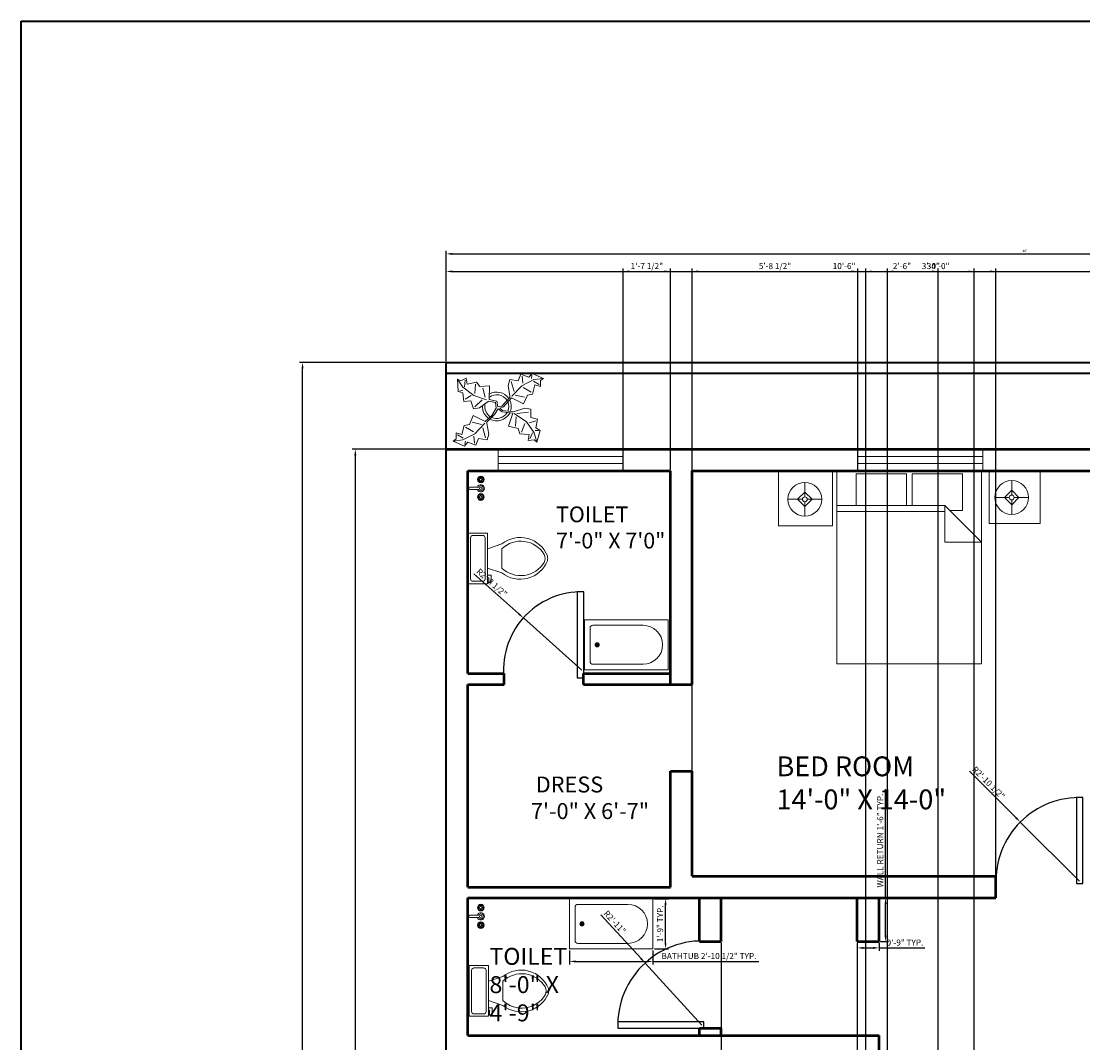
# Model space of a CAD drawing. Units: inches. Extents: x 65 to 818, y -87 to 880.
# Tile 5 of 6: x 65 to 505, y 457 to 880. Entities that reach past the tile are written whole.
import ezdxf

# ---------------------------------------------------------------- set-up
doc = ezdxf.new("R2010")
doc.units = ezdxf.units.IN
for name, color, linetype, lineweight in [('A-ANNO-DIMS', 2, 'Continuous', 18), ('A-ANNO-TTLB', 7, 'Continuous', 35), ('A-AREA-IDEN', 7, 'Continuous', 25), ('A-DOOR', 3, 'Continuous', 25), ('A-FLOR-FIXT', 9, 'Continuous', 18), ('A-FURN', 8, 'Continuous', 18), ('A-GLAZ', 4, 'Continuous', 18), ('A-WALL', 7, 'Continuous', 50), ('C-PROP', 7, 'Continuous', 35), ('E-LITE', 2, 'Continuous', 18), ('L-PLNT', 94, 'Continuous', 13)]:
    doc.layers.add(name, color=color, linetype=linetype, lineweight=lineweight)
doc.styles.get("Standard").update_dxf_attribs({"font": 'arial.ttf'})
doc.dimstyles.new('ISO-25', dxfattribs={"dimtxt": 2.5, "dimasz": 2.5, "dimexe": 1.25, "dimexo": 0.625, "dimtad": 1, "dimtxsty": 'Standard', "dimcen": 2.5, "dimadec": 0, "dimazin": 0, "dimtfac": 1, "dimtmove": 0, "dimatfit": 3, "dimfxl": 1, "dimarcsym": 0})

# ---------------------------------------------------------------- blocks, each defined once
blk = doc.blocks.new('Bed - Queen')
for p, q in [((0, -80.00003), (0, 0)), ((0, 0), (59.99999, 0)), ((59.99999, 0), (59.99999, -80.00003)), ((7.99999, -1.2), (28.79998, -1.2)), ((7.99999, -14.4), (7.99999, -1.2)), ((28.79998, -1.2), (28.79998, -14.4)), ((31.19999, -1.2), (51.99999, -1.2)), ((31.19999, -14.4), (31.19999, -1.2)), ((51.99999, -1.2), (51.99999, -16.4)), ((0, -14.4), (44.8, -14.4)), ((44.8, -16.8), (0, -16.8)), ((59.99999, -29.6), (44.8, -14.4)), ((44.8, -14.4), (44.8, -29.6)), ((51.99999, -16.4), (46.79936, -16.4)), ((44.8, -29.6), (59.99999, -29.6)), ((59.99999, -80.00003), (0, -80.00003))]:
    blk.add_line(p, q)
blk = doc.blocks.new('Toilet - top')
for p, q in [((9.5, -6), (9.5, -2)), ((-10, -8.5), (-8, -8.5)), ((-10, -9.5), (-10, -8.5)), ((-8, -8.5), (-8, -8)), ((-7, -8), (-7, -9.5)), ((-4, -8), (-6, -14)), ((4, -8), (6, -14)), ((-7, -9.5), (-10, -9.5)), ((4, -14), (-4, -14))]:
    blk.add_line(p, q)
blk.add_lwpolyline([(10.5, -8), (10.5, 0), (-10.5, 0), (-10.5, -8)], close=True)
for points in [[(-9.5, -2), (-9.5, -6)], [(8.5, -1), (-8.5, -1)], [(-8.5, -7), (8.5, -7)]]:
    blk.add_lwpolyline(points)
for centre, radius, start, end in [((-8.62, -1.88), 0.884, 81.8699, 188.1301), ((8.62, -1.88), 0.884, 351.8699, 98.1301), ((-8.62, -6.12), 0.884, 171.8699, 278.1301), ((8.62, -6.12), 0.884, 261.8699, 8.1301), ((3.52, -21.58), 12.17, 141.4691, 247.9714), ((4.2, -21.82), 11.33, 136.3677, 238.9468), ((-3.52, -21.58), 12.17, 292.0284, 38.5307), ((-4.2, -21.82), 11.33, 301.053, 43.6321), ((0, -27.88), 4, 245.7318, 294.2682), ((0, -29), 4, 254.8605, 285.1395)]:
    blk.add_arc(centre, radius, start, end)
blk = doc.blocks.new('Bath Tub - 26 x 60 in.')
for p, q in [((8, -18), (10, -18)), ((9, -17), (9, -19))]:
    blk.add_line(p, q)
blk.add_lwpolyline([(0, -36), (0, 0), (60, 0), (60, -36)], close=True)
for points in [[(4, -30), (4, -6)], [(6, -4), (42, -4)], [(42, -32), (6, -32)]]:
    blk.add_lwpolyline(points)
for radius in [1.5, 1]:
    blk.add_circle((9, -18), radius)
for centre, radius, start, end in [((5.75, -5.75), 1.77, 81.8699, 188.1301), ((42, -18), 14, 270, 90), ((5.75, -30.25), 1.77, 171.8699, 278.1301)]:
    blk.add_arc(centre, radius, start, end)
blk = doc.blocks.new('Faucet - Bathroom top')
for p, q in [((-4.107, 0.125), (-4.375, 0.125)), ((-3.75, 0.4788), (-3.75, 0.75)), ((-3.5, 0.482), (-3.5, 0.75)), ((-3.1461, 0.125), (-2.875, 0.125)), ((3.143, 0.125), (2.875, 0.125)), ((3.5, 0.4788), (3.5, 0.75)), ((3.75, 0.482), (3.75, 0.75)), ((4.1039, 0.125), (4.375, 0.125)), ((-4.1039, -0.125), (-4.375, -0.125)), ((-3.75, -0.4821), (-3.75, -0.75)), ((-3.5, -0.4789), (-3.5, -0.75)), ((-3.143, -0.125), (-2.875, -0.125)), ((-0.5, -0.8639), (-0.5, -4.5)), ((0.5, -4.5), (0.5, -0.8631)), ((3.1461, -0.125), (2.875, -0.125)), ((3.5, -0.4821), (3.5, -0.75)), ((3.75, -0.4789), (3.75, -0.75)), ((4.107, -0.125), (4.375, -0.125))]:
    blk.add_line(p, q)
for centre, radius in [((-3.625, 0), 1.375), ((-4.625, 0), 0.2795), ((-3.625, 0), 0.5), ((-3.625, 1), 0.2795), ((-2.625, 0), 0.2795), ((0, 0), 0.5), ((3.625, 0), 1.375), ((2.625, 0), 0.2795), ((3.625, 0), 0.5), ((3.625, 1), 0.2795), ((4.625, 0), 0.2795), ((-3.625, -1), 0.2795), ((3.625, -1), 0.2795)]:
    blk.add_circle(centre, radius)
for centre, radius, start, end in [((-3.625, 0), 1, 105.2407, 164.2093), ((-3.625, 0), 1, 16.44125, 74.07887), ((0, 0), 1.5, 289.6514, 250.3603), ((0, 0), 1, 300.3431, 239.7554), ((3.625, 0), 1, 106.12, 164.0884), ((3.625, 0), 1, 16.23422, 73.90469), ((-3.625, 0), 1, 196.2342, 253.9047), ((-3.625, 0), 1, 286.12, 344.0884), ((3.625, 0), 1, 196.4413, 254.0789), ((3.625, 0), 1, 285.2407, 344.2093), ((0, -4.5), 0.5, 180, 0)]:
    blk.add_arc(centre, radius, start, end)
blk = doc.blocks.new('Plant - Rubber or Philodendron')
for p, q in [((8.8871, 10.7908), (9.9809, 13.4933)), ((9.9809, 13.4933), (13.3837, 12.301)), ((13.3837, 12.301), (14.68, 13.9039)), ((14.68, 13.9039), (19.3848, 11.8146)), ((-16.2005, 11.4774), (-13.9899, 8.1064)), ((-16.2005, 11.4774), (-14.8639, 10.7964)), ((-16.0159, 6.3329), (-16.2005, 11.4774)), ((-14.8639, 10.7964), (-12.6195, 11.8975)), ((-13.3174, 8.325), (-13.0735, 11.0065)), ((-12.6195, 11.8975), (-12.1909, 9.4345)), ((-12.1909, 9.4345), (-8.3829, 10.3)), ((-8.8369, 9.409), (-9.0894, 5.6095)), ((-8.3829, 10.3), (-7.0549, 8.501)), ((4.6914, 8.8812), (5.3859, 11.2828)), ((4.6914, 8.8812), (5.5014, 4.4831)), ((5.3859, 11.2828), (8.8871, 10.7908)), ((5.9878, 10.4842), (7.1971, 6.3869)), ((15.3859, 11.3055), (10.3916, 8.7942)), ((10.5828, 12.6946), (10.8893, 9.7953)), ((14.5816, 13.2037), (14.3848, 11.8033)), ((15.7909, 9.1065), (14.8995, 5.3044)), ((15.2875, 10.6053), (17.5907, 9.2105)), ((19.3848, 11.8146), (15.3859, 11.3055)), ((18.1925, 8.4119), (15.7909, 9.1065)), ((19.3848, 11.8146), (18.1868, 10.9119)), ((18.1868, 10.9119), (18.1925, 8.4119)), ((-14.0069, 5.8704), (-16.0159, 6.3329)), ((-15.3434, 6.5514), (-13.9984, 6.9884)), ((-13.5868, 2.2894), (-14.0069, 5.8704)), ((-13.9899, 8.1064), (-9.5434, 4.7185)), ((-13.1329, 3.1804), (-10.6614, 4.727)), ((-9.5434, 4.7185), (-4.1917, 2.9888)), ((-7.0549, 8.501), (-3.0284, 8.6941)), ((-4.8529, 4.012), (-5.7184, 7.82)), ((-3.0284, 8.6941), (-3.0709, 3.1041)), ((5.4346, 3.9146), (5.5014, 4.4831)), ((10.3916, 8.7942), (6.2847, 4.4028)), ((7.7005, 4.8881), (11.5025, 3.9967)), ((14.2977, 6.1031), (10.9934, 7.9956)), ((12.7005, 4.8994), (11.1089, 1.1958)), ((14.8995, 5.3044), (12.7005, 4.8994)), ((-10.6784, 2.491), (-13.5868, 2.2894)), ((-9.5858, -0.8715), (-10.6784, 2.491)), ((-9.1318, 0.0195), (-5.9793, 2.9025)), ((-7.1228, -0.443), (-3.5248, 2.2131)), ((-3.5248, 2.2131), (-3.3011, 2.4355)), ((-3.3011, 2.4355), (-0.5306, 1.7947)), ((-3.0709, 3.1041), (0.0797, 2.3163)), ((-0.5306, 1.7947), (-0.2255, -0.5527)), ((-0.5306, 1.7947), (-0.5306, 1.7947)), ((0.0797, 2.3163), (0.4866, -0.031)), ((0.4866, -0.031), (2.1141, 0.2298)), ((2.1141, 0.2298), (5.4346, 3.9146)), ((6.1032, 3.6844), (2.8262, -0.031)), ((11.1089, 1.1958), (6.1032, 3.6844)), ((-11.3237, -7.2629), (-9.7321, -3.5593)), ((-9.7321, -3.5593), (-4.7264, -6.0479)), ((-7.1228, -0.443), (-9.5858, -0.8715)), ((-2.019, -3.6148), (-4.7264, -6.0479)), ((-4.0579, -6.2781), (-0.9375, -3.1608)), ((-2.019, -3.6148), (-0.2255, -0.5527)), ((-0.9375, -3.1608), (0.5883, -0.8135)), ((0.5883, -0.8135), (2.2447, -2.0916)), ((2.8262, -0.031), (1.3003, -0.5527)), ((1.3003, -0.5527), (2.4193, -1.4655)), ((2.2447, -2.0916), (6.7108, -2.6626)), ((2.4193, -1.4655), (6.895, -2.1175)), ((4.943, -7.9659), (6.7108, -2.6626)), ((11.6605, -0.5413), (6.895, -2.1175)), ((12.3677, -6.1981), (7.219, -2.6772)), ((8.125, -4.0768), (7.7715, -7.9659)), ((8.3544, -2.7453), (13.1973, -2.1704)), ((11.6605, -0.5413), (14.1354, -0.8948)), ((14.1354, -0.8948), (14.1354, -4.4304)), ((-14.4141, -11.4699), (-13.5228, -7.6679)), ((-13.5228, -7.6679), (-11.3237, -7.2629)), ((-12.921, -8.4665), (-9.6166, -10.359)), ((-6.3237, -7.2516), (-10.1257, -6.3602)), ((-9.0148, -11.1577), (-4.9047, -6.8122)), ((-4.611, -12.8477), (-5.8203, -8.7504)), ((-4.1246, -6.8466), (-4.0579, -6.2781)), ((-3.3146, -11.2447), (-4.1246, -6.8466)), ((8.8321, -9.0266), (4.943, -7.9659)), ((10.2463, -10.4408), (11.6605, -6.9053)), ((15.5496, -10.7943), (12.3677, -6.1981)), ((16.2567, -5.8446), (13.4283, -6.5517)), ((14.1354, -4.4304), (16.9638, -5.1375)), ((16.9638, -5.1375), (16.2567, -8.673)), ((16.2567, -8.673), (18.0245, -9.7337)), ((-16.8157, -10.7754), (-14.4141, -11.4699)), ((-16.8101, -13.2754), (-16.8157, -10.7754)), ((-13.9107, -12.9688), (-16.2139, -11.574)), ((-14.0091, -13.669), (-9.0148, -11.1577)), ((-9.206, -15.0581), (-9.5126, -12.1588)), ((-7.5103, -13.1543), (-8.6042, -15.8568)), ((-4.0092, -13.6463), (-7.5103, -13.1543)), ((-3.3146, -11.2447), (-4.0092, -13.6463)), ((9.5392, -11.1479), (8.8321, -9.0266)), ((13.4283, -11.5015), (9.5392, -11.1479)), ((13.0748, -13.9763), (13.4283, -11.5015)), ((14.8425, -10.7943), (13.7819, -13.2692)), ((16.6103, -14.6834), (15.5496, -10.7943)), ((17.3174, -9.7337), (15.9032, -9.7337)), ((18.0245, -9.7337), (16.6103, -14.6834)), ((-18.008, -14.1781), (-16.8101, -13.2754)), ((-18.008, -14.1781), (-14.0091, -13.669)), ((-13.3032, -16.2674), (-18.008, -14.1781)), ((-12.0069, -14.6645), (-13.3032, -16.2674)), ((-13.2048, -15.5672), (-13.008, -14.1668)), ((-8.6042, -15.8568), (-12.0069, -14.6645)), ((15.5496, -13.6228), (13.0748, -13.9763)), ((16.6103, -14.6834), (15.5496, -13.6228))]:
    blk.add_line(p, q)
for centre, radius, start, end in [((0, 0), 6.1275, 34.37569, 120.1028), ((-0.0601, -0.2075), 5.2461, 33.82192, 124.9414), ((0.0308, 0.1664), 6, 178.6147, 235.1169), ((0.0308, 0.1664), 5, 168.1647, 238.6725), ((-0.2664, 0.1682), 5.2775, 338.4094, 20.03007), ((-0.098, 0.1364), 6.1288, 341.2017, 26.09184), ((-0.0234, 0.3825), 6.1492, 242.5812, 331.2714), ((-0.1102, 0.4886), 5.2883, 247.3711, 327.472)]:
    blk.add_arc(centre, radius, start, end)
blk = doc.blocks.new('Lamp - Table')
for p, q in [((0, 7), (0, 1)), ((-1, 0), (-7, 0)), ((0, 3), (-3, 0)), ((-3, 0), (0, -3)), ((3, 0), (0, 3)), ((0, -3), (3, 0)), ((1, 0), (7, 0)), ((0, -1), (0, -7))]:
    blk.add_line(p, q)
for radius in [7, 1]:
    blk.add_circle((0, 0), radius)
blk = doc.blocks.new('*D13')
at = {"layer": 'A-ANNO-DIMS', "color": 0, "lineweight": -2, "transparency": 16777216}
for p, q in [((240.8, 739.67), (240.8, 785.28)), ((243.3, 784.03), (718.3, 784.03)), ((720.8, 739.67), (720.8, 785.28))]:
    blk.add_line(p, q, dxfattribs=at)
at = {"layer": 'A-ANNO-DIMS', "color": 0, "transparency": 16777216}
for points in [[(243.3, 784.45), (243.3, 783.61), (240.8, 784.03)], [(718.3, 784.45), (718.3, 783.61), (720.8, 784.03)]]:
    blk.add_solid(points, dxfattribs=at)
at = {"layer": 'Defpoints', "color": 0, "transparency": 16777216}
for p in [(720.8, 784.03), (240.8, 739.04), (720.8, 739.04)]:
    blk.add_point(p, dxfattribs=at)
at = {"layer": 'A-ANNO-DIMS', "color": 0, "transparency": 16777216, "insert": (480.8, 785.17), "char_height": 1, "attachment_point": 5}
blk.add_mtext("40'", dxfattribs=at)
blk = doc.blocks.new('*D14')
at = {"layer": 'A-ANNO-DIMS', "color": 0, "lineweight": -2, "transparency": 16777216}
for p, q in [((240.17, 739.04), (179.98, 739.04)), ((181.23, 21.54), (181.23, 736.54)), ((240.17, 19.04), (179.98, 19.04))]:
    blk.add_line(p, q, dxfattribs=at)
at = {"layer": 'A-ANNO-DIMS', "color": 0, "transparency": 16777216}
for points in [[(180.81, 736.54), (181.65, 736.54), (181.23, 739.04)], [(180.81, 21.54), (181.65, 21.54), (181.23, 19.04)]]:
    blk.add_solid(points, dxfattribs=at)
at = {"layer": 'Defpoints', "color": 0, "transparency": 16777216}
for p in [(181.23, 739.04), (240.8, 739.04), (240.8, 19.04)]:
    blk.add_point(p, dxfattribs=at)
at = {"layer": 'A-ANNO-DIMS', "color": 0, "transparency": 16777216, "insert": (180.09, 379.04), "char_height": 1, "attachment_point": 5, "rotation": 90}
blk.add_mtext("60'", dxfattribs=at)
blk = doc.blocks.new('WIN-52X9-PLAN')
for p, q in [((9, 51.82), (0, 51.82)), ((0, 51.82), (0, 0)), ((3, 0), (3, 51.82)), ((6, 51.82), (6, 0)), ((9, 0), (9, 51.82)), ((0, 0), (9, 0))]:
    blk.add_line(p, q)
blk = doc.blocks.new('WALL-RETURN-9X18')
for p, q in [((0, 0), (0, 18)), ((9, 0), (9, 18)), ((0, 0), (9, 0))]:
    blk.add_line(p, q)
blk = doc.blocks.new('DOOR-LEAF-36-NOM')
blk.add_lwpolyline([(0, 0), (2.67, 0), (2.67, 35.67), (0, 35.67)], close=True)
blk = doc.blocks.new('*D32')
at = {"layer": 'A-ANNO-DIMS', "color": 0, "lineweight": -2, "transparency": 16777216}
for p, q in [((291.94, 495.3), (291.94, 489.49)), ((326.56, 495.3), (326.56, 489.49)), ((294.44, 490.74), (324.06, 490.74)), ((326.56, 490.74), (370.48, 490.74))]:
    blk.add_line(p, q, dxfattribs=at)
at = {"layer": 'A-ANNO-DIMS', "color": 0, "transparency": 16777216}
for points in [[(294.44, 491.15), (294.44, 490.32), (291.94, 490.74)], [(324.06, 491.15), (324.06, 490.32), (326.56, 490.74)]]:
    blk.add_solid(points, dxfattribs=at)
at = {"layer": 'Defpoints', "color": 0, "transparency": 16777216}
for p in [(291.94, 495.93), (326.56, 495.93), (326.56, 490.74)]:
    blk.add_point(p, dxfattribs=at)
at = {"layer": 'A-ANNO-DIMS', "color": 0, "transparency": 16777216, "insert": (349.77, 492.65), "char_height": 2.5, "attachment_point": 5}
blk.add_mtext('BATHTUB 2\'-10 1/2" TYP.', dxfattribs=at)
blk = doc.blocks.new('*D33')
at = {"layer": 'A-ANNO-DIMS', "color": 0, "lineweight": -2, "transparency": 16777216}
for p, q in [((327.18, 516.7), (333, 516.7)), ((331.75, 498.43), (331.75, 514.2)), ((327.18, 495.93), (333, 495.93))]:
    blk.add_line(p, q, dxfattribs=at)
at = {"layer": 'A-ANNO-DIMS', "color": 0, "transparency": 16777216}
for points in [[(331.34, 514.2), (332.17, 514.2), (331.75, 516.7)], [(331.34, 498.43), (332.17, 498.43), (331.75, 495.93)]]:
    blk.add_solid(points, dxfattribs=at)
at = {"layer": 'Defpoints', "color": 0, "transparency": 16777216}
for p in [(326.56, 516.7), (331.75, 516.7), (326.56, 495.93)]:
    blk.add_point(p, dxfattribs=at)
at = {"layer": 'A-ANNO-DIMS', "color": 0, "transparency": 16777216, "insert": (329.85, 506.31), "char_height": 2.5, "attachment_point": 5, "rotation": 90}
blk.add_mtext('1\'-9" TYP.', dxfattribs=at)
blk = doc.blocks.new('*D40')
at = {"layer": 'A-ANNO-DIMS', "color": 0, "lineweight": -2, "transparency": 16777216}
for p, q in [((423, 517.04), (423, 562.13)), ((420.92, 517.04), (424.25, 517.04)), ((423, 501.54), (423, 514.54)), ((420.92, 499.04), (424.25, 499.04))]:
    blk.add_line(p, q, dxfattribs=at)
at = {"layer": 'A-ANNO-DIMS', "color": 0, "transparency": 16777216}
for points in [[(422.58, 514.54), (423.42, 514.54), (423, 517.04)], [(422.58, 501.54), (423.42, 501.54), (423, 499.04)]]:
    blk.add_solid(points, dxfattribs=at)
at = {"layer": 'Defpoints', "color": 0, "transparency": 16777216}
for p in [(420.3, 517.04), (423, 517.04), (420.3, 499.04)]:
    blk.add_point(p, dxfattribs=at)
at = {"layer": 'A-ANNO-DIMS', "color": 0, "transparency": 16777216, "insert": (421.1, 540.84), "char_height": 2.5, "attachment_point": 5, "rotation": 90}
blk.add_mtext('WALL RETURN 1\'-6" TYP.', dxfattribs=at)
blk = doc.blocks.new('*D41')
at = {"layer": 'A-ANNO-DIMS', "color": 0, "lineweight": -2, "transparency": 16777216}
for p, q in [((411.3, 498.42), (411.3, 495.09)), ((420.3, 498.42), (420.3, 495.09)), ((413.8, 496.34), (417.8, 496.34)), ((420.3, 496.34), (439.29, 496.34))]:
    blk.add_line(p, q, dxfattribs=at)
at = {"layer": 'A-ANNO-DIMS', "color": 0, "transparency": 16777216}
for points in [[(413.8, 496.76), (413.8, 495.92), (411.3, 496.34)], [(417.8, 496.76), (417.8, 495.92), (420.3, 496.34)]]:
    blk.add_solid(points, dxfattribs=at)
at = {"layer": 'Defpoints', "color": 0, "transparency": 16777216}
for p in [(411.3, 499.04), (420.3, 499.04), (420.3, 496.34)]:
    blk.add_point(p, dxfattribs=at)
at = {"layer": 'A-ANNO-DIMS', "color": 0, "transparency": 16777216, "insert": (431.04, 498.24), "char_height": 2.5, "attachment_point": 5}
blk.add_mtext('0\'-9" TYP.', dxfattribs=at)
blk = doc.blocks.new('*D48')
at = {"layer": 'A-ANNO-DIMS', "color": 0, "lineweight": -2, "transparency": 16777216}
for p, q in [((342.8, 526.67), (342.8, 777.99)), ((345.3, 776.74), (466.3, 776.74)), ((468.8, 526.67), (468.8, 777.99))]:
    blk.add_line(p, q, dxfattribs=at)
at = {"layer": 'A-ANNO-DIMS', "color": 0, "transparency": 16777216}
for points in [[(345.3, 777.16), (345.3, 776.32), (342.8, 776.74)], [(466.3, 777.16), (466.3, 776.32), (468.8, 776.74)]]:
    blk.add_solid(points, dxfattribs=at)
at = {"layer": 'Defpoints', "color": 0, "transparency": 16777216}
for p in [(468.8, 776.74), (342.8, 526.04), (468.8, 526.04)]:
    blk.add_point(p, dxfattribs=at)
at = {"layer": 'A-ANNO-DIMS', "color": 0, "transparency": 16777216, "insert": (405.8, 778.64), "char_height": 2.5, "attachment_point": 5}
blk.add_mtext('10\'-6"', dxfattribs=at)
blk = doc.blocks.new('*D50')
at = {"layer": 'A-ANNO-DIMS', "color": 0, "lineweight": -2, "transparency": 16777216}
for p, q in [((240.8, 703.67), (240.8, 777.99)), ((243.3, 776.74), (646.3, 776.74)), ((648.8, 703.67), (648.8, 777.99))]:
    blk.add_line(p, q, dxfattribs=at)
at = {"layer": 'A-ANNO-DIMS', "color": 0, "transparency": 16777216}
for points in [[(243.3, 777.16), (243.3, 776.32), (240.8, 776.74)], [(646.3, 777.16), (646.3, 776.32), (648.8, 776.74)]]:
    blk.add_solid(points, dxfattribs=at)
at = {"layer": 'Defpoints', "color": 0, "transparency": 16777216}
for p in [(648.8, 776.74), (240.8, 703.04), (648.8, 703.04)]:
    blk.add_point(p, dxfattribs=at)
at = {"layer": 'A-ANNO-DIMS', "color": 0, "transparency": 16777216, "insert": (444.8, 778.64), "char_height": 2.5, "attachment_point": 5}
blk.add_mtext('34\'-0"', dxfattribs=at)
blk = doc.blocks.new('*D52')
at = {"layer": 'A-ANNO-DIMS', "color": 0, "lineweight": -2, "transparency": 16777216}
for p, q in [((240.17, 703.04), (201.85, 703.04)), ((203.1, 700.54), (203.1, 95.54)), ((249.17, 93.04), (201.85, 93.04))]:
    blk.add_line(p, q, dxfattribs=at)
at = {"layer": 'A-ANNO-DIMS', "color": 0, "transparency": 16777216}
for points in [[(202.68, 700.54), (203.52, 700.54), (203.1, 703.04)], [(202.68, 95.54), (203.52, 95.54), (203.1, 93.04)]]:
    blk.add_solid(points, dxfattribs=at)
at = {"layer": 'Defpoints', "color": 0, "transparency": 16777216}
for p in [(240.8, 703.04), (203.1, 93.04), (249.8, 93.04)]:
    blk.add_point(p, dxfattribs=at)
at = {"layer": 'A-ANNO-DIMS', "color": 0, "transparency": 16777216, "insert": (201.2, 398.04), "char_height": 2.5, "attachment_point": 5, "rotation": 90}
blk.add_mtext('50\'-10"', dxfattribs=at)
blk = doc.blocks.new('*D58')
at = {"layer": 'A-ANNO-DIMS', "color": 0, "lineweight": -2, "transparency": 16777216}
for p, q in [((414.8, 238.17), (414.8, 777.99)), ((417.3, 776.74), (442.3, 776.74)), ((444.8, 238.17), (444.8, 777.99))]:
    blk.add_line(p, q, dxfattribs=at)
at = {"layer": 'A-ANNO-DIMS', "color": 0, "transparency": 16777216}
for points in [[(417.3, 777.16), (417.3, 776.32), (414.8, 776.74)], [(442.3, 777.16), (442.3, 776.32), (444.8, 776.74)]]:
    blk.add_solid(points, dxfattribs=at)
at = {"layer": 'Defpoints', "color": 0, "transparency": 16777216}
for p in [(444.8, 776.74), (414.8, 237.54), (444.8, 237.54)]:
    blk.add_point(p, dxfattribs=at)
at = {"layer": 'A-ANNO-DIMS', "color": 0, "transparency": 16777216, "insert": (429.8, 778.64), "char_height": 2.5, "attachment_point": 5}
blk.add_mtext('2\'-6"', dxfattribs=at)
blk = doc.blocks.new('*D61')
at = {"layer": 'A-ANNO-DIMS', "color": 0, "lineweight": -2, "transparency": 16777216}
for p, q in [((314.22, 694.7), (314.22, 777.99)), ((316.72, 776.74), (331.3, 776.74)), ((333.8, 694.67), (333.8, 777.99))]:
    blk.add_line(p, q, dxfattribs=at)
at = {"layer": 'A-ANNO-DIMS', "color": 0, "transparency": 16777216}
for points in [[(316.72, 777.16), (316.72, 776.32), (314.22, 776.74)], [(331.3, 777.16), (331.3, 776.32), (333.8, 776.74)]]:
    blk.add_solid(points, dxfattribs=at)
at = {"layer": 'Defpoints', "color": 0, "transparency": 16777216}
for p in [(333.8, 776.74), (314.22, 694.08), (333.8, 694.04)]:
    blk.add_point(p, dxfattribs=at)
at = {"layer": 'A-ANNO-DIMS', "color": 0, "transparency": 16777216, "insert": (324.01, 778.66), "char_height": 2.5, "attachment_point": 5}
blk.add_mtext('1\'-7 1/2"', dxfattribs=at)
blk = doc.blocks.new('*D62')
at = {"layer": 'A-ANNO-DIMS', "color": 0, "lineweight": -2, "transparency": 16777216}
for p, q in [((342.8, 694.67), (342.8, 777.99)), ((345.3, 776.74), (409, 776.74)), ((411.5, 694.72), (411.5, 777.99))]:
    blk.add_line(p, q, dxfattribs=at)
at = {"layer": 'A-ANNO-DIMS', "color": 0, "transparency": 16777216}
for points in [[(345.3, 777.16), (345.3, 776.32), (342.8, 776.74)], [(409, 777.16), (409, 776.32), (411.5, 776.74)]]:
    blk.add_solid(points, dxfattribs=at)
at = {"layer": 'Defpoints', "color": 0, "transparency": 16777216}
for p in [(411.5, 776.74), (342.8, 694.04), (411.5, 694.09)]:
    blk.add_point(p, dxfattribs=at)
at = {"layer": 'A-ANNO-DIMS', "color": 0, "transparency": 16777216, "insert": (377.15, 778.66), "char_height": 2.5, "attachment_point": 5}
blk.add_mtext('5\'-8 1/2"', dxfattribs=at)
blk = doc.blocks.new('*D66')
at = {"layer": 'A-ANNO-DIMS', "color": 0, "lineweight": -2, "transparency": 16777216}
for p, q in [((423.8, 320.67), (423.8, 777.99)), ((426.3, 776.74), (457.3, 776.74)), ((459.8, 320.67), (459.8, 777.99))]:
    blk.add_line(p, q, dxfattribs=at)
at = {"layer": 'A-ANNO-DIMS', "color": 0, "transparency": 16777216}
for points in [[(426.3, 777.16), (426.3, 776.32), (423.8, 776.74)], [(457.3, 777.16), (457.3, 776.32), (459.8, 776.74)]]:
    blk.add_solid(points, dxfattribs=at)
at = {"layer": 'Defpoints', "color": 0, "transparency": 16777216}
for p in [(459.8, 776.74), (423.8, 320.04), (459.8, 320.04)]:
    blk.add_point(p, dxfattribs=at)
at = {"layer": 'A-ANNO-DIMS', "color": 0, "transparency": 16777216, "insert": (441.8, 778.64), "char_height": 2.5, "attachment_point": 5}
blk.add_mtext('3\'-0"', dxfattribs=at)
blk = doc.blocks.new('*D72')
at = {"layer": 'A-ANNO-DIMS', "color": 0, "lineweight": -2, "transparency": 16777216}
for p, q in [((354.8, 498.42), (354.8, -19.91)), ((411.3, 498.42), (411.3, -19.91)), ((357.3, -18.66), (408.8, -18.66))]:
    blk.add_line(p, q, dxfattribs=at)
at = {"layer": 'A-ANNO-DIMS', "color": 0, "transparency": 16777216}
for points in [[(357.3, -18.25), (357.3, -19.08), (354.8, -18.66)], [(408.8, -18.25), (408.8, -19.08), (411.3, -18.66)]]:
    blk.add_solid(points, dxfattribs=at)
at = {"layer": 'Defpoints', "color": 0, "transparency": 16777216}
for p in [(354.8, 499.04), (411.3, 499.04), (411.3, -18.66)]:
    blk.add_point(p, dxfattribs=at)
at = {"layer": 'A-ANNO-DIMS', "color": 0, "transparency": 16777216, "insert": (383.05, -16.75), "char_height": 2.5, "attachment_point": 5}
blk.add_mtext('4\'-8 1/2"', dxfattribs=at)
blk = doc.blocks.new('*D75')
at = {"layer": 'A-ANNO-DIMS', "color": 0, "lineweight": -2, "transparency": 16777216}
for p, q in [((304.99, 510.04), (321.59, 491.91)), ((346.88, 464.29), (323.28, 490.07))]:
    blk.add_line(p, q, dxfattribs=at)
at = {"layer": 'A-ANNO-DIMS', "color": 0, "transparency": 16777216}
blk.add_solid([(321.9, 492.19), (321.29, 491.63), (323.28, 490.07)], dxfattribs=at)
at = {"layer": 'Defpoints', "color": 0, "transparency": 16777216}
for p in [(323.28, 490.07), (346.88, 464.29)]:
    blk.add_point(p, dxfattribs=at)
at = {"layer": 'A-ANNO-DIMS', "color": 0, "transparency": 16777216, "insert": (310.51, 506.8), "char_height": 2.5, "attachment_point": 5, "rotation": 312.4716}
blk.add_mtext('R2\'-11"', dxfattribs=at)
blk = doc.blocks.new('*D76')
at = {"layer": 'A-ANNO-DIMS', "color": 0, "lineweight": -2, "transparency": 16777216}
for p, q in [((457.78, 569.59), (477.11, 550.3)), ((503.39, 524.06), (478.88, 548.53))]:
    blk.add_line(p, q, dxfattribs=at)
at = {"layer": 'A-ANNO-DIMS', "color": 0, "transparency": 16777216}
blk.add_solid([(477.4, 550.59), (476.81, 550), (478.88, 548.53)], dxfattribs=at)
at = {"layer": 'Defpoints', "color": 0, "transparency": 16777216}
for p in [(478.88, 548.53), (503.39, 524.06)]:
    blk.add_point(p, dxfattribs=at)
at = {"layer": 'A-ANNO-DIMS', "color": 0, "transparency": 16777216, "insert": (465.52, 564.57), "char_height": 2.5, "attachment_point": 5, "rotation": 315.05}
blk.add_mtext('R2\'-10 1/2"', dxfattribs=at)
blk = doc.blocks.new('*D79')
at = {"layer": 'A-ANNO-DIMS', "color": 0, "lineweight": -2, "transparency": 16777216}
for p, q in [((252.23, 651.45), (270.92, 634.78)), ((297.03, 611.49), (272.79, 633.12))]:
    blk.add_line(p, q, dxfattribs=at)
at = {"layer": 'A-ANNO-DIMS', "color": 0, "transparency": 16777216}
blk.add_solid([(271.2, 635.09), (270.64, 634.47), (272.79, 633.12)], dxfattribs=at)
at = {"layer": 'Defpoints', "color": 0, "transparency": 16777216}
for p in [(272.79, 633.12), (297.03, 611.49)]:
    blk.add_point(p, dxfattribs=at)
at = {"layer": 'A-ANNO-DIMS', "color": 0, "transparency": 16777216, "insert": (259.51, 647.52), "char_height": 2.5, "attachment_point": 5, "rotation": 318.2701}
blk.add_mtext('R2\'-8 1/2"', dxfattribs=at)

msp = doc.modelspace()

# ---------------------------------------------------------------- linework, layer by layer
at = {"layer": 'A-ANNO-TTLB'}
msp.add_lwpolyline([(64.55, 880.46), (817.59, 880.46), (817.59, -87.37), (64.55, -87.37)], close=True, dxfattribs=at)
at = {"layer": 'A-DOOR'}
for centre, radius, start, end in [((297.03, 611.49), 32.49, 88.6401, 187.9006), ((503.39, 524.06), 34.63, 87.6679, 182.4337), ((346.88, 464.29), 34.94, 82.8651, 182.079)]:
    msp.add_arc(centre, radius, start, end, dxfattribs=at)
at = {"layer": 'A-FURN'}
for points in [[(378.6, 693.9), (400.95, 693.9), (400.95, 671.27), (378.6, 671.27)], [(465.91, 693.84), (487.17, 693.84), (487.17, 672.22), (465.91, 672.22)]]:
    msp.add_lwpolyline(points, close=True, dxfattribs=at)
at = {"layer": 'A-WALL'}
for p, q in [((240.8, 703.04), (648.8, 703.04)), ((249.8, 694.04), (333.8, 694.04)), ((249.8, 610.04), (249.8, 694.04)), ((333.8, 605.54), (333.8, 694.04)), ((342.8, 694.04), (510.8, 694.04)), ((342.8, 605.54), (342.8, 694.04)), ((249.8, 610.04), (264.8, 610.04)), ((264.8, 605.54), (264.8, 610.04)), ((297.8, 605.54), (297.8, 610.04)), ((297.8, 610.04), (333.8, 610.04)), ((249.8, 605.54), (264.8, 605.54)), ((249.8, 521.54), (249.8, 605.54)), ((297.8, 605.54), (342.8, 605.54)), ((333.8, 521.54), (333.8, 569.54)), ((333.8, 569.54), (342.8, 569.54)), ((342.8, 526.04), (342.8, 569.54)), ((342.8, 526.04), (468.8, 526.04)), ((468.8, 517.04), (468.8, 526.04)), ((249.8, 521.54), (333.8, 521.54)), ((249.8, 517.04), (468.8, 517.04)), ((249.8, 460.04), (249.8, 517.04)), ((342.8, 517.04), (468.8, 517.04)), ((345.8, 460.04), (345.8, 463.04)), ((345.8, 463.04), (354.8, 463.04)), ((354.8, 460.04), (354.8, 463.04)), ((249.8, 460.04), (420.3, 460.04)), ((420.3, 361.04), (420.3, 460.04))]:
    msp.add_line(p, q, dxfattribs=at)
at = {"layer": 'C-PROP'}
for p, q in [((240.8, 19.04), (240.8, 739.04)), ((240.8, 739.04), (720.8, 739.04)), ((240.8, 734.54), (716.3, 734.54))]:
    msp.add_line(p, q, dxfattribs=at)

# ---------------------------------------------------------------- block references
at = {"layer": 'A-DOOR'}
for p in [(295.15, 608.28), (502.13, 523)]:
    msp.add_blockref('DOOR-LEAF-36-NOM', p, dxfattribs=at)
at = {"layer": 'A-DOOR', "rotation": 90.00000000000003}
msp.add_blockref('DOOR-LEAF-36-NOM', (347.63, 463.03), dxfattribs=at)
at = {"layer": 'A-FLOR-FIXT'}
for name, p, rotation in [('Faucet - Bathroom top', (255.13, 686.87), 270), ('Toilet - top', (249.91, 657.81), 90), ('Faucet - Bathroom top', (255.13, 509.41), 270), ('Toilet - top', (250.32, 478.52), 90)]:
    msp.add_blockref(name, p, dxfattribs=dict(at, rotation=rotation))
at = {"layer": 'A-FLOR-FIXT', "xscale": 0.5769824704091256, "yscale": 0.5769824704091256, "zscale": 0.5769824704091256}
for p in [(298.21, 632.37), (291.94, 516.7)]:
    msp.add_blockref('Bath Tub - 26 x 60 in.', p, dxfattribs=at)
at = {"layer": 'A-FURN'}
msp.add_blockref('Bed - Queen', (402.86, 694.09), dxfattribs=at)
at = {"layer": 'A-GLAZ'}
for p, rotation in [((262.4, 703.08), 270), ((411.5, 703.09), 269.9999999999999)]:
    msp.add_blockref('WIN-52X9-PLAN', p, dxfattribs=dict(at, rotation=rotation))
at = {"layer": 'A-WALL'}
for p in [(345.8, 499.04), (411.3, 499.04)]:
    msp.add_blockref('WALL-RETURN-9X18', p, dxfattribs=at)
at = {"layer": 'E-LITE'}
for p in [(389.52, 682.31), (475.32, 683.06)]:
    msp.add_blockref('Lamp - Table', p, dxfattribs=at)
at = {"layer": 'L-PLNT'}
msp.add_blockref('Plant - Rubber or Philodendron', (261.75, 720.61), dxfattribs=at)

# ---------------------------------------------------------------- texts
at = {"layer": 'A-AREA-IDEN', "attachment_point": 1}
for s, width, gutter_width, insert, char_height in [('TOILET\\P7\'-0" X 7\'0"', 79.1197, 32.64, (286.34, 679.32), 6.5286), ('BED ROOM\\P14\'-0" X 14-0"', 223.4994, 41.1, (377.8, 575.72), 8.2202), (' DRESS\\P7\'-0" X 6\'-7"', 92.9101, 33.05, (275.91, 567.39), 6.6099), ('TOILET\\P8\'-0" X 4\'-9"', 50.7506, 35.13, (258.75, 496.36), 7.0261)]:
    msp.add_mtext_dynamic_manual_height_columns(s, width=width, gutter_width=gutter_width, heights=[0], dxfattribs=dict(at, insert=insert, char_height=char_height))

# ---------------------------------------------------------------- dimensions: what is measured, and where the dimension line sits
at = {"layer": 'A-ANNO-DIMS'}
for base, p1, p2, override, picture, middle in [((720.8, 784.03), (240.8, 739.04), (720.8, 739.04), {"dimtxt": 1, "dimdec": 0, "dimlunit": 3, "dimclrd": 0, "dimclre": 0, "dimclrt": 0, "dimtdec": 0}, '*D13', (480.8, 785.17)), ((648.8, 776.74), (240.8, 703.04), (648.8, 703.04), {"dimdec": 1, "dimlfac": 1, "dimrnd": 0, "dimzin": 1, "dimdsep": 46, "dimlunit": 4, "dimfrac": 2}, '*D50', (444.8, 778.64)), ((333.8, 776.74), (314.22, 694.08), (333.8, 694.04), {"dimdec": 1, "dimlfac": 1, "dimrnd": 0, "dimzin": 1, "dimdsep": 46, "dimlunit": 4, "dimfrac": 2}, '*D61', (324.01, 778.66)), ((411.5, 776.74), (342.8, 694.04), (411.5, 694.09), {"dimdec": 1, "dimlfac": 1, "dimrnd": 0, "dimzin": 1, "dimdsep": 46, "dimlunit": 4, "dimfrac": 2}, '*D62', (377.15, 778.66)), ((468.8, 776.74), (342.8, 526.04), (468.8, 526.04), {"dimdec": 1, "dimlfac": 1, "dimrnd": 0, "dimzin": 1, "dimdsep": 46, "dimlunit": 4, "dimfrac": 2}, '*D48', (405.8, 778.64)), ((444.8, 776.74), (414.8, 237.54), (444.8, 237.54), {"dimdec": 1, "dimlfac": 1, "dimrnd": 0, "dimzin": 1, "dimdsep": 46, "dimlunit": 4, "dimfrac": 2}, '*D58', (429.8, 778.64)), ((459.8, 776.74), (423.8, 320.04), (459.8, 320.04), {"dimdec": 1, "dimlfac": 1, "dimrnd": 0, "dimzin": 1, "dimdsep": 46, "dimlunit": 4, "dimfrac": 2}, '*D66', (441.8, 778.64)), ((411.3, -18.66), (354.8, 499.04), (411.3, 499.04), {"dimdec": 1, "dimlfac": 1, "dimrnd": 0, "dimzin": 1, "dimdsep": 46, "dimlunit": 4, "dimfrac": 2}, '*D72', (383.05, -16.75))]:
    dim = msp.add_linear_dim(base=base, p1=p1, p2=p2, dimstyle='ISO-25', override=override, dxfattribs=at)
    dim.commit()
    dim.dimension.update_dxf_attribs({"geometry": picture, "text_midpoint": middle})
for base, p1, p2, override, picture, middle in [((181.23, 739.04), (240.8, 19.04), (240.8, 739.04), {"dimtxt": 1, "dimdec": 0, "dimlunit": 3, "dimclrd": 0, "dimclre": 0, "dimclrt": 0, "dimtdec": 0}, '*D14', (180.09, 379.04)), ((203.1, 93.04), (240.8, 703.04), (249.8, 93.04), {"dimdec": 1, "dimlfac": 1, "dimrnd": 0, "dimzin": 1, "dimdsep": 46, "dimlunit": 4, "dimfrac": 2}, '*D52', (201.2, 398.04))]:
    dim = msp.add_linear_dim(base=base, p1=p1, p2=p2, angle=90, dimstyle='ISO-25', override=override, dxfattribs=at)
    dim.commit()
    dim.dimension.update_dxf_attribs({"geometry": picture, "text_midpoint": middle})
for center, mpoint, picture, middle in [((297.03, 611.49), (272.79, 633.12), '*D79', (258.24, 646.09)), ((503.39, 524.06), (478.88, 548.53), '*D76', (464.17, 563.21)), ((346.876, 464.292), (323.2809, 490.0671), '*D75', (309.1239, 505.5321))]:
    dim = msp.add_radius_dim(center=center, mpoint=mpoint, dimstyle='ISO-25', override={"dimdec": 1, "dimlfac": 1, "dimrnd": 0, "dimzin": 1, "dimdsep": 46, "dimlunit": 4, "dimfrac": 2}, dxfattribs=at)
    dim.commit()
    dim.dimension.update_dxf_attribs({"geometry": picture, "text_midpoint": middle, "dimtype": 164})
for base, p1, p2, text, picture, middle in [((423, 517.04), (420.3, 499.04), (420.3, 517.04), 'WALL RETURN <> TYP.', '*D40', (421.1, 540.84)), ((331.75, 516.7), (326.56, 495.93), (326.56, 516.7), '<> TYP.', '*D33', (329.85, 506.31))]:
    dim = msp.add_linear_dim(base=base, p1=p1, p2=p2, angle=90, text=text, dimstyle='ISO-25', override={"dimdec": 1, "dimlfac": 1, "dimrnd": 0, "dimzin": 1, "dimdsep": 46, "dimlunit": 4, "dimfrac": 2}, dxfattribs=at)
    dim.commit()
    dim.dimension.update_dxf_attribs({"geometry": picture, "text_midpoint": middle})
for base, p1, p2, text, picture, middle in [((420.3, 496.34), (411.3, 499.04), (420.3, 499.04), '<> TYP.', '*D41', (431.04, 498.24)), ((326.56, 490.74), (291.94, 495.93), (326.56, 495.93), 'BATHTUB <> TYP.', '*D32', (349.77, 492.65))]:
    dim = msp.add_linear_dim(base=base, p1=p1, p2=p2, text=text, dimstyle='ISO-25', override={"dimdec": 1, "dimlfac": 1, "dimrnd": 0, "dimzin": 1, "dimdsep": 46, "dimlunit": 4, "dimfrac": 2}, dxfattribs=at)
    dim.commit()
    dim.dimension.update_dxf_attribs({"geometry": picture, "text_midpoint": middle})

doc.saveas('drawing.dxf')
